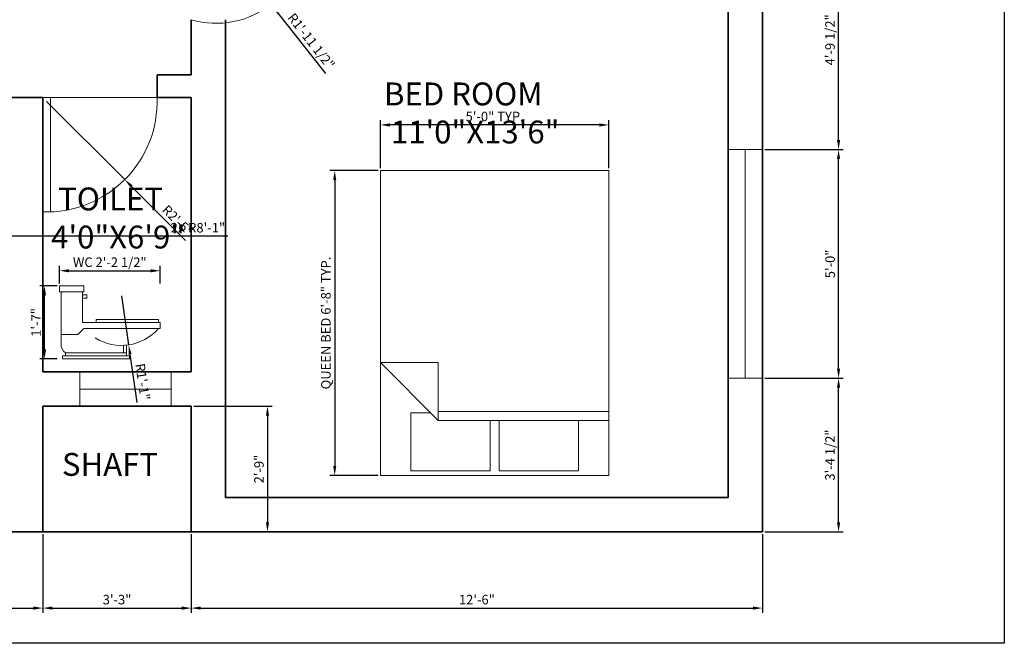
# Model space of a CAD drawing. Units: inches. Extents: x 5717 to 6221, y 11359 to 11763.
# Tile 3 of 4: x 5963 to 6221, y 11382 to 11546. Entities that reach past the tile are written whole.
import ezdxf

# ---------------------------------------------------------------- set-up
doc = ezdxf.new("R2010")
doc.units = ezdxf.units.IN
for name, color, linetype, lineweight, true_color in [('A-ANNO-DIMS', 254, 'Continuous', 13, 0xfeeab9), ('A-ANNO-TTLB', 51, 'Continuous', 25, 0xf8f6b0), ('A-AREA-IDEN', 11, 'Continuous', 20, 0xf27172), ('A-WALL', 244, 'Continuous', 35, 0x991b1e)]:
    doc.layers.add(name, color=color, linetype=linetype, lineweight=lineweight, true_color=true_color)
for name, color, linetype, lineweight in [('A-DOOR', 5, 'Continuous', 18), ('A-FLOR-FIXT', 1, 'Continuous', 18), ('A-FURN', 8, 'Continuous', 18), ('A-GLAZ', 4, 'Continuous', 18)]:
    doc.layers.add(name, color=color, linetype=linetype, lineweight=lineweight)
doc.styles.get("Standard").update_dxf_attribs({"font": 'arial.ttf'})
doc.dimstyles.new('ISO-25', dxfattribs={"dimtxt": 2.5, "dimasz": 2.5, "dimexe": 1.25, "dimexo": 0.625, "dimtad": 1, "dimlunit": 3, "dimtxsty": 'Standard', "dimcen": 2.5, "dimadec": 0, "dimazin": 0, "dimtfac": 1, "dimtmove": 0, "dimatfit": 3, "dimfxl": 1, "dimarcsym": 0})

# ---------------------------------------------------------------- blocks, each defined once
blk = doc.blocks.new('Toilet - side')
for p, q in [((0.5, 5), (0.5, 22)), ((7.5, 22), (7.5, 12)), ((7.5, 21), (9, 21)), ((9, 20), (7.5, 20)), ((9, 21), (9, 20)), ((32.5, 13), (12, 13)), ((12, 13), (12, 12)), ((32.5, 12), (32.5, 13)), ((8, 10), (6, 8)), ((7.5, 12), (33, 12)), ((33, 10), (8, 10)), ((33, 12), (33, 10)), ((6, 8), (0.5, 8)), ((21, 4.5), (21, 2)), ((22, 2), (22, 4.54)), ((22, 2), (2, 2)), ((2, 2), (2, 1)), ((22, 1), (22, 2))]:
    blk.add_line(p, q)
for points in [[(0, 22), (0, 24), (8, 24), (8, 22)], [(1, 0), (1, 1), (23, 1), (23, 0)]]:
    blk.add_lwpolyline(points, close=True)
for centre, radius, start, end in [((20.3, 20.7), 16.23, 238.1872, 318.7702), ((3.75, 4.75), 3.26, 175.6013, 237.5288)]:
    blk.add_arc(centre, radius, start, end)
blk = doc.blocks.new('Bed - Queen')
for p, q in [((0, -80.00003), (0, 0)), ((0, 0), (59.99999, 0)), ((59.99999, 0), (59.99999, -80.00003)), ((7.99999, -1.2), (28.79998, -1.2)), ((7.99999, -14.4), (7.99999, -1.2)), ((28.79998, -1.2), (28.79998, -14.4)), ((31.19999, -1.2), (51.99999, -1.2)), ((31.19999, -14.4), (31.19999, -1.2)), ((51.99999, -1.2), (51.99999, -16.4)), ((0, -14.4), (44.8, -14.4)), ((59.99999, -29.6), (44.8, -14.4)), ((44.8, -14.4), (44.8, -29.6)), ((44.8, -16.8), (0, -16.8)), ((51.99999, -16.4), (46.79936, -16.4)), ((44.8, -29.6), (59.99999, -29.6)), ((59.99999, -80.00003), (0, -80.00003))]:
    blk.add_line(p, q)
blk = doc.blocks.new('DOOR-LEAF-30IN')
for p, q in [((2, 30), (0, 30)), ((0, 30), (0, 0)), ((2, 0), (2, 30))]:
    blk.add_line(p, q)
blk = doc.blocks.new('WIN-24IN')
for p, q in [((0, 9), (0, 0)), ((24, 9), (0, 9)), ((24, 9), (24, 0)), ((24, 0), (24, 9)), ((0, 4.5), (24, 4.5)), ((0, 0), (24, 0))]:
    blk.add_line(p, q)
blk = doc.blocks.new('*D20')
at = {"layer": 'A-ANNO-DIMS', "color": 0, "lineweight": -2, "transparency": 16777216}
for p, q in [((6056.94, 11505.95), (6044.32, 11505.95)), ((6045.57, 11503.45), (6045.57, 11428.45)), ((6056.94, 11425.95), (6044.32, 11425.95))]:
    blk.add_line(p, q, dxfattribs=at)
at = {"layer": 'A-ANNO-DIMS', "color": 0, "transparency": 16777216}
for points in [[(6045.15, 11503.45), (6045.98, 11503.45), (6045.57, 11505.95)], [(6045.15, 11428.45), (6045.98, 11428.45), (6045.57, 11425.95)]]:
    blk.add_solid(points, dxfattribs=at)
at = {"layer": 'Defpoints', "color": 0, "transparency": 16777216}
for p in [(6057.57, 11505.95), (6045.57, 11425.95), (6057.57, 11425.95)]:
    blk.add_point(p, dxfattribs=at)
at = {"layer": 'A-ANNO-DIMS', "color": 0, "transparency": 16777216, "insert": (6043.57, 11465.95), "char_height": 2.5, "attachment_point": 5, "rotation": 90}
blk.add_mtext('QUEEN BED 6\'-8" TYP.', dxfattribs=at)
blk = doc.blocks.new('*D21')
at = {"layer": 'A-ANNO-DIMS', "color": 0, "lineweight": -2, "transparency": 16777216}
for p, q in [((6057.57, 11506.58), (6057.57, 11519.2)), ((6117.57, 11506.58), (6117.57, 11519.2)), ((6115.07, 11517.95), (6060.07, 11517.95))]:
    blk.add_line(p, q, dxfattribs=at)
at = {"layer": 'A-ANNO-DIMS', "color": 0, "transparency": 16777216}
for points in [[(6060.07, 11518.37), (6060.07, 11517.53), (6057.57, 11517.95)], [(6115.07, 11518.37), (6115.07, 11517.53), (6117.57, 11517.95)]]:
    blk.add_solid(points, dxfattribs=at)
at = {"layer": 'Defpoints', "color": 0, "transparency": 16777216}
for p in [(6057.57, 11517.95), (6057.57, 11505.95), (6117.57, 11505.95)]:
    blk.add_point(p, dxfattribs=at)
at = {"layer": 'A-ANNO-DIMS', "color": 0, "transparency": 16777216, "insert": (6087.57, 11519.85), "char_height": 2.5, "attachment_point": 5}
blk.add_mtext('5\'-0" TYP.', dxfattribs=at)
blk = doc.blocks.new('*D28')
at = {"layer": 'A-ANNO-DIMS', "color": 0, "lineweight": -2, "transparency": 16777216}
for p, q in [((5973.29, 11476.33), (5973.29, 11480.92)), ((5975.79, 11479.67), (5997.19, 11479.67)), ((5999.69, 11476.33), (5999.69, 11480.92))]:
    blk.add_line(p, q, dxfattribs=at)
at = {"layer": 'A-ANNO-DIMS', "color": 0, "transparency": 16777216}
for points in [[(5975.79, 11480.08), (5975.79, 11479.25), (5973.29, 11479.67)], [(5997.19, 11480.08), (5997.19, 11479.25), (5999.69, 11479.67)]]:
    blk.add_solid(points, dxfattribs=at)
at = {"layer": 'Defpoints', "color": 0, "transparency": 16777216}
for p in [(5999.69, 11479.67), (5973.29, 11475.71), (5999.69, 11475.71)]:
    blk.add_point(p, dxfattribs=at)
at = {"layer": 'A-ANNO-DIMS', "color": 0, "transparency": 16777216, "insert": (5986.49, 11481.58), "char_height": 2.5, "attachment_point": 5}
blk.add_mtext('WC 2\'-2 1/2"', dxfattribs=at)
blk = doc.blocks.new('*D29')
at = {"layer": 'A-ANNO-DIMS', "color": 0, "lineweight": -2, "transparency": 16777216}
for p, q in [((5972.67, 11475.71), (5968.08, 11475.71)), ((5969.33, 11459.01), (5969.33, 11473.21)), ((5972.67, 11456.51), (5968.08, 11456.51))]:
    blk.add_line(p, q, dxfattribs=at)
at = {"layer": 'A-ANNO-DIMS', "color": 0, "transparency": 16777216}
for points in [[(5968.92, 11473.21), (5969.75, 11473.21), (5969.33, 11475.71)], [(5968.92, 11459.01), (5969.75, 11459.01), (5969.33, 11456.51)]]:
    blk.add_solid(points, dxfattribs=at)
at = {"layer": 'Defpoints', "color": 0, "transparency": 16777216}
for p in [(5969.33, 11475.71), (5973.29, 11475.71), (5973.29, 11456.51)]:
    blk.add_point(p, dxfattribs=at)
at = {"layer": 'A-ANNO-DIMS', "color": 0, "transparency": 16777216, "insert": (5967.45, 11466.11), "char_height": 2.5, "attachment_point": 5, "rotation": 90}
blk.add_mtext('1\'-7"', dxfattribs=at)
blk = doc.blocks.new('*D38')
at = {"layer": 'A-ANNO-DIMS', "color": 0, "lineweight": -2, "transparency": 16777216}
for p, q in [((5797.9, 11410.48), (5797.9, 11389.86)), ((5968.9, 11410.48), (5968.9, 11389.86)), ((5800.4, 11391.11), (5966.4, 11391.11))]:
    blk.add_line(p, q, dxfattribs=at)
at = {"layer": 'A-ANNO-DIMS', "color": 0, "transparency": 16777216}
for points in [[(5800.4, 11391.53), (5800.4, 11390.69), (5797.9, 11391.11)], [(5966.4, 11391.53), (5966.4, 11390.69), (5968.9, 11391.11)]]:
    blk.add_solid(points, dxfattribs=at)
at = {"layer": 'Defpoints', "color": 0, "transparency": 16777216}
for p in [(5797.9, 11411.11), (5968.9, 11411.11), (5968.9, 11391.11)]:
    blk.add_point(p, dxfattribs=at)
at = {"layer": 'A-ANNO-DIMS', "color": 0, "transparency": 16777216, "insert": (5883.4, 11393.01), "char_height": 2.5, "attachment_point": 5}
blk.add_mtext('14\'-3"', dxfattribs=at)
blk = doc.blocks.new('*D39')
at = {"layer": 'A-ANNO-DIMS', "color": 0, "lineweight": -2, "transparency": 16777216}
for p, q in [((5968.9, 11410.48), (5968.9, 11389.86)), ((6007.9, 11410.48), (6007.9, 11389.86)), ((5971.4, 11391.11), (6005.4, 11391.11))]:
    blk.add_line(p, q, dxfattribs=at)
at = {"layer": 'A-ANNO-DIMS', "color": 0, "transparency": 16777216}
for points in [[(5971.4, 11391.53), (5971.4, 11390.69), (5968.9, 11391.11)], [(6005.4, 11391.53), (6005.4, 11390.69), (6007.9, 11391.11)]]:
    blk.add_solid(points, dxfattribs=at)
at = {"layer": 'Defpoints', "color": 0, "transparency": 16777216}
for p in [(5968.9, 11411.11), (6007.9, 11411.11), (6007.9, 11391.11)]:
    blk.add_point(p, dxfattribs=at)
at = {"layer": 'A-ANNO-DIMS', "color": 0, "transparency": 16777216, "insert": (5988.4, 11393.01), "char_height": 2.5, "attachment_point": 5}
blk.add_mtext('3\'-3"', dxfattribs=at)
blk = doc.blocks.new('*D40')
at = {"layer": 'A-ANNO-DIMS', "color": 0, "lineweight": -2, "transparency": 16777216}
for p, q in [((6007.9, 11410.48), (6007.9, 11389.86)), ((6157.9, 11410.48), (6157.9, 11389.86)), ((6010.4, 11391.11), (6155.4, 11391.11))]:
    blk.add_line(p, q, dxfattribs=at)
at = {"layer": 'A-ANNO-DIMS', "color": 0, "transparency": 16777216}
for points in [[(6010.4, 11391.53), (6010.4, 11390.69), (6007.9, 11391.11)], [(6155.4, 11391.53), (6155.4, 11390.69), (6157.9, 11391.11)]]:
    blk.add_solid(points, dxfattribs=at)
at = {"layer": 'Defpoints', "color": 0, "transparency": 16777216}
for p in [(6007.9, 11411.11), (6157.9, 11411.11), (6157.9, 11391.11)]:
    blk.add_point(p, dxfattribs=at)
at = {"layer": 'A-ANNO-DIMS', "color": 0, "transparency": 16777216, "insert": (6082.9, 11393.01), "char_height": 2.5, "attachment_point": 5}
blk.add_mtext('12\'-6"', dxfattribs=at)
blk = doc.blocks.new('*D41')
at = {"layer": 'A-ANNO-DIMS', "color": 0, "lineweight": -2, "transparency": 16777216}
for p, q in [((6158.53, 11451.47), (6179.15, 11451.47)), ((6177.9, 11413.61), (6177.9, 11448.97)), ((6158.53, 11411.11), (6179.15, 11411.11))]:
    blk.add_line(p, q, dxfattribs=at)
at = {"layer": 'A-ANNO-DIMS', "color": 0, "transparency": 16777216}
for points in [[(6177.49, 11448.97), (6178.32, 11448.97), (6177.9, 11451.47)], [(6177.49, 11413.61), (6178.32, 11413.61), (6177.9, 11411.11)]]:
    blk.add_solid(points, dxfattribs=at)
at = {"layer": 'Defpoints', "color": 0, "transparency": 16777216}
for p in [(6157.9, 11451.47), (6177.9, 11451.47), (6157.9, 11411.11)]:
    blk.add_point(p, dxfattribs=at)
at = {"layer": 'A-ANNO-DIMS', "color": 0, "transparency": 16777216, "insert": (6175.98, 11431.29), "char_height": 2.5, "attachment_point": 5, "rotation": 90}
blk.add_mtext('3\'-4 1/2"', dxfattribs=at)
blk = doc.blocks.new('*D42')
at = {"layer": 'A-ANNO-DIMS', "color": 0, "lineweight": -2, "transparency": 16777216}
for p, q in [((6158.53, 11511.47), (6179.15, 11511.47)), ((6177.9, 11453.97), (6177.9, 11508.97)), ((6158.53, 11451.47), (6179.15, 11451.47))]:
    blk.add_line(p, q, dxfattribs=at)
at = {"layer": 'A-ANNO-DIMS', "color": 0, "transparency": 16777216}
for points in [[(6177.49, 11508.97), (6178.32, 11508.97), (6177.9, 11511.47)], [(6177.49, 11453.97), (6178.32, 11453.97), (6177.9, 11451.47)]]:
    blk.add_solid(points, dxfattribs=at)
at = {"layer": 'Defpoints', "color": 0, "transparency": 16777216}
for p in [(6157.9, 11511.47), (6177.9, 11511.47), (6157.9, 11451.47)]:
    blk.add_point(p, dxfattribs=at)
at = {"layer": 'A-ANNO-DIMS', "color": 0, "transparency": 16777216, "insert": (6176, 11481.47), "char_height": 2.5, "attachment_point": 5, "rotation": 90}
blk.add_mtext('5\'-0"', dxfattribs=at)
blk = doc.blocks.new('*D43')
at = {"layer": 'A-ANNO-DIMS', "color": 0, "lineweight": -2, "transparency": 16777216}
for p, q in [((6158.53, 11569.11), (6179.15, 11569.11)), ((6177.9, 11513.97), (6177.9, 11566.61)), ((6158.53, 11511.47), (6179.15, 11511.47))]:
    blk.add_line(p, q, dxfattribs=at)
at = {"layer": 'A-ANNO-DIMS', "color": 0, "transparency": 16777216}
for points in [[(6177.49, 11566.61), (6178.32, 11566.61), (6177.9, 11569.11)], [(6177.49, 11513.97), (6178.32, 11513.97), (6177.9, 11511.47)]]:
    blk.add_solid(points, dxfattribs=at)
at = {"layer": 'Defpoints', "color": 0, "transparency": 16777216}
for p in [(6157.9, 11569.11), (6177.9, 11569.11), (6157.9, 11511.47)]:
    blk.add_point(p, dxfattribs=at)
at = {"layer": 'A-ANNO-DIMS', "color": 0, "transparency": 16777216, "insert": (6175.98, 11540.29), "char_height": 2.5, "attachment_point": 5, "rotation": 90}
blk.add_mtext('4\'-9 1/2"', dxfattribs=at)
blk = doc.blocks.new('*D57')
at = {"layer": 'A-ANNO-DIMS', "color": 0, "lineweight": -2, "transparency": 16777216}
for p, q in [((6008.53, 11444.11), (6029.15, 11444.11)), ((6027.9, 11441.61), (6027.9, 11413.61)), ((6008.53, 11411.11), (6029.15, 11411.11))]:
    blk.add_line(p, q, dxfattribs=at)
at = {"layer": 'A-ANNO-DIMS', "color": 0, "transparency": 16777216}
for points in [[(6027.49, 11441.61), (6028.32, 11441.61), (6027.9, 11444.11)], [(6027.49, 11413.61), (6028.32, 11413.61), (6027.9, 11411.11)]]:
    blk.add_solid(points, dxfattribs=at)
at = {"layer": 'Defpoints', "color": 0, "transparency": 16777216}
for p in [(6007.9, 11444.11), (6007.9, 11411.11), (6027.9, 11411.11)]:
    blk.add_point(p, dxfattribs=at)
at = {"layer": 'A-ANNO-DIMS', "color": 0, "transparency": 16777216, "insert": (6026, 11427.61), "char_height": 2.5, "attachment_point": 5, "rotation": 90}
blk.add_mtext('2\'-9"', dxfattribs=at)
blk = doc.blocks.new('*D64')
at = {"layer": 'A-ANNO-DIMS', "color": 0, "lineweight": -2, "transparency": 16777216}
for p, q in [((5969.9, 11524.11), (5990.42, 11503.59)), ((6006.37, 11487.64), (5992.19, 11501.82))]:
    blk.add_line(p, q, dxfattribs=at)
at = {"layer": 'A-ANNO-DIMS', "color": 0, "transparency": 16777216}
blk.add_solid([(5992.48, 11502.12), (5991.89, 11501.53), (5990.42, 11503.59)], dxfattribs=at)
at = {"layer": 'Defpoints', "color": 0, "transparency": 16777216}
for p in [(5969.9, 11524.11), (5990.42, 11503.59)]:
    blk.add_point(p, dxfattribs=at)
at = {"layer": 'A-ANNO-DIMS', "color": 0, "transparency": 16777216, "insert": (6004.08, 11492.62), "char_height": 2.5, "attachment_point": 5, "rotation": 315.0011}
blk.add_mtext('R2\'-5"', dxfattribs=at)
blk = doc.blocks.new('*D66')
at = {"layer": 'A-ANNO-DIMS', "color": 0, "lineweight": -2, "transparency": 16777216}
for p, q in [((6014.46, 11568.11), (6028.94, 11549.64)), ((6043.2, 11531.46), (6030.48, 11547.68))]:
    blk.add_line(p, q, dxfattribs=at)
at = {"layer": 'A-ANNO-DIMS', "color": 0, "transparency": 16777216}
blk.add_solid([(6030.81, 11547.93), (6030.16, 11547.42), (6028.94, 11549.64)], dxfattribs=at)
at = {"layer": 'Defpoints', "color": 0, "transparency": 16777216}
for p in [(6014.46, 11568.11), (6028.94, 11549.64)]:
    blk.add_point(p, dxfattribs=at)
at = {"layer": 'A-ANNO-DIMS', "color": 0, "transparency": 16777216, "insert": (6039.14, 11539.75), "char_height": 2.5, "attachment_point": 5, "rotation": 308.1145}
blk.add_mtext('R1\'-11 1/2"', dxfattribs=at)
blk = doc.blocks.new('*D67')
at = {"layer": 'A-ANNO-DIMS', "color": 0, "lineweight": -2, "transparency": 16777216}
for p, q in [((5854.49, 11488.73), (5951.44, 11488.73)), ((6017.47, 11488.73), (5953.94, 11488.73))]:
    blk.add_line(p, q, dxfattribs=at)
at = {"layer": 'A-ANNO-DIMS', "color": 0, "transparency": 16777216}
blk.add_solid([(5953.94, 11489.15), (5953.94, 11488.32), (5951.44, 11488.73)], dxfattribs=at)
at = {"layer": 'Defpoints', "color": 0, "transparency": 16777216}
for p in [(5854.49, 11488.73), (5951.44, 11488.73)]:
    blk.add_point(p, dxfattribs=at)
at = {"layer": 'A-ANNO-DIMS', "color": 0, "transparency": 16777216, "insert": (6009.62, 11490.64), "char_height": 2.5, "attachment_point": 5, "rotation": 360}
blk.add_mtext('2X R8\'-1"', dxfattribs=at)
blk = doc.blocks.new('*D69')
at = {"layer": 'A-ANNO-DIMS', "color": 0, "lineweight": -2, "transparency": 16777216}
for p, q in [((5989.53, 11473.06), (5991.44, 11460.22)), ((5993.7, 11445.1), (5991.81, 11457.75))]:
    blk.add_line(p, q, dxfattribs=at)
at = {"layer": 'A-ANNO-DIMS', "color": 0, "transparency": 16777216}
blk.add_solid([(5992.22, 11457.81), (5991.4, 11457.69), (5991.44, 11460.22)], dxfattribs=at)
at = {"layer": 'Defpoints', "color": 0, "transparency": 16777216}
for p in [(5989.53, 11473.06), (5991.44, 11460.22)]:
    blk.add_point(p, dxfattribs=at)
at = {"layer": 'A-ANNO-DIMS', "color": 0, "transparency": 16777216, "insert": (5994.8, 11450.47), "char_height": 2.5, "attachment_point": 5, "rotation": 278.4771}
blk.add_mtext('R1\'-1"', dxfattribs=at)

msp = doc.modelspace()

# ---------------------------------------------------------------- linework, layer by layer
at = {"layer": 'A-ANNO-TTLB'}
msp.add_lwpolyline([(5717.423, 11763.126), (6221.432, 11763.126), (6221.432, 11381.867), (5717.423, 11381.867)], close=True, dxfattribs=at)
at = {"layer": 'A-DOOR'}
for p, q in [((5968.902, 11525.109), (5998.902, 11525.109)), ((5998.902, 11525.109), (5968.902, 11525.109))]:
    msp.add_line(p, q, dxfattribs=at)
for centre, radius, start, end in [((6014.455, 11568.109), 23.469, 253.78655, 2.44213), ((5969.902, 11524.109), 29.017, 268.02507, 1.97493)]:
    msp.add_arc(centre, radius, start, end, dxfattribs=at)
at = {"layer": 'A-GLAZ'}
for p, q in [((6148.902, 11451.47), (6148.902, 11511.47)), ((6157.902, 11511.47), (6148.902, 11511.47)), ((6153.402, 11451.47), (6153.402, 11511.47)), ((6157.902, 11451.47), (6157.902, 11511.47)), ((6148.902, 11451.47), (6157.902, 11451.47))]:
    msp.add_line(p, q, dxfattribs=at)
at = {"layer": 'A-WALL'}
for p, q in [((6157.902, 11411.109), (6157.902, 11711.109)), ((6148.902, 11420.109), (6148.902, 11569.109)), ((6007.902, 11531.109), (6007.902, 11545.574)), ((6016.902, 11420.109), (6016.902, 11545.574)), ((5998.902, 11531.109), (6007.902, 11531.109)), ((5998.902, 11525.109), (5998.902, 11531.109)), ((5959.902, 11525.109), (5968.902, 11525.109)), ((5968.902, 11453.109), (5968.902, 11525.109)), ((5998.902, 11525.109), (6007.902, 11525.109)), ((6007.902, 11453.109), (6007.902, 11525.109)), ((5968.902, 11453.109), (6007.902, 11453.109)), ((5968.902, 11411.109), (5968.902, 11444.109)), ((5968.902, 11444.109), (6007.902, 11444.109)), ((6007.902, 11411.109), (6007.902, 11444.109)), ((6016.902, 11420.109), (6148.902, 11420.109)), ((5797.902, 11411.109), (6157.902, 11411.109))]:
    msp.add_line(p, q, dxfattribs=at)

# ---------------------------------------------------------------- block references
at = {"layer": 'A-DOOR', "rotation": 180}
msp.add_blockref('DOOR-LEAF-30IN', (5970.902, 11525.109), dxfattribs=at)
at = {"layer": 'A-FLOR-FIXT', "xscale": 0.8, "yscale": 0.8, "zscale": 0.8}
msp.add_blockref('Toilet - side', (5973.293, 11456.506), dxfattribs=at)
at = {"layer": 'A-FURN', "rotation": 180}
msp.add_blockref('Bed - Queen', (6117.568, 11425.95), dxfattribs=at)
at = {"layer": 'A-GLAZ'}
msp.add_blockref('WIN-24IN', (5978.601, 11444.109), dxfattribs=at)

# ---------------------------------------------------------------- texts
at = {"layer": 'A-AREA-IDEN', "char_height": 6, "attachment_point": 1}
for s, insert in [('     BED ROOM\\P      11\'0"X13\'6"', (6049.33, 11529.088)), (' TOILET\\P4\'0"X6\'9"', (5971.091, 11501.517)), ('  SHAFT', (5970.26, 11431.829))]:
    msp.add_mtext_dynamic_manual_height_columns(s, width=116.60264, gutter_width=12.5, heights=[0], dxfattribs=dict(at, insert=insert))

# ---------------------------------------------------------------- dimensions: what is measured, and where the dimension line sits
at = {"layer": 'A-ANNO-DIMS'}
for center, mpoint, picture, middle in [((6014.455, 11568.109), (6028.941, 11549.644), '*D66', (6037.632, 11538.566)), ((5969.902, 11524.109), (5990.421, 11503.591), '*D64', (6002.732, 11491.28))]:
    dim = msp.add_radius_dim(center=center, mpoint=mpoint, dimstyle='ISO-25', override={"dimdec": 1, "dimlfac": 1, "dimrnd": 0, "dimzin": 1, "dimdsep": 46, "dimlunit": 4, "dimfrac": 2}, dxfattribs=at)
    dim.commit()
    dim.dimension.update_dxf_attribs({"geometry": picture, "text_midpoint": middle, "dimtype": 164})
for base, p1, p2, angle, picture, middle in [((6177.902, 11569.109), (6157.902, 11511.47), (6157.902, 11569.109), 90, '*D43', (6175.985, 11540.29)), ((6177.902, 11511.47), (6157.902, 11451.47), (6157.902, 11511.47), 90, '*D42', (6176.001, 11481.47)), ((5969.333, 11475.706), (5973.293, 11456.506), (5973.293, 11475.706), 90, '*D29', (5967.453, 11466.106)), ((6177.902, 11451.47), (6157.902, 11411.109), (6157.902, 11451.47), 90, '*D41', (6175.984, 11431.29)), ((6027.902, 11411.109), (6007.902, 11444.109), (6007.902, 11411.109), 270, '*D57', (6026.001, 11427.609))]:
    dim = msp.add_linear_dim(base=base, p1=p1, p2=p2, angle=angle, dimstyle='ISO-25', override={"dimdec": 1, "dimlfac": 1, "dimrnd": 0, "dimzin": 1, "dimdsep": 46, "dimlunit": 4, "dimfrac": 2}, dxfattribs=at)
    dim.commit()
    dim.dimension.update_dxf_attribs({"geometry": picture, "text_midpoint": middle})
for base, p1, p2, angle, text, picture, middle in [((6057.568, 11517.95), (6117.568, 11505.95), (6057.568, 11505.95), 180, '<> TYP.', '*D21', (6087.568, 11519.852)), ((6045.568, 11425.95), (6057.568, 11505.95), (6057.568, 11425.95), 270, 'QUEEN BED <> TYP.', '*D20', (6043.573, 11465.95))]:
    dim = msp.add_linear_dim(base=base, p1=p1, p2=p2, angle=angle, text=text, dimstyle='ISO-25', override={"dimdec": 1, "dimlfac": 1, "dimrnd": 0, "dimzin": 1, "dimdsep": 46, "dimlunit": 4, "dimfrac": 2}, dxfattribs=at)
    dim.commit()
    dim.dimension.update_dxf_attribs({"geometry": picture, "text_midpoint": middle})
dim = msp.add_radius_dim(center=(5854.485, 11488.735), mpoint=(5951.443, 11488.735), text='2X <>', dimstyle='ISO-25', override={"dimdec": 1, "dimlfac": 1, "dimrnd": 0, "dimzin": 1, "dimdsep": 46, "dimlunit": 4, "dimfrac": 2}, dxfattribs=at)
dim.commit()
dim.dimension.update_dxf_attribs({"geometry": '*D67', "text_midpoint": (6009.617, 11488.735), "dimtype": 164})
dim = msp.add_linear_dim(base=(5999.693, 11479.666), p1=(5973.293, 11475.706), p2=(5999.693, 11475.706), text='WC <>', dimstyle='ISO-25', override={"dimdec": 1, "dimlfac": 1, "dimrnd": 0, "dimzin": 1, "dimdsep": 46, "dimlunit": 4, "dimfrac": 2}, dxfattribs=at)
dim.commit()
dim.dimension.update_dxf_attribs({"geometry": '*D28', "text_midpoint": (5986.493, 11481.583)})
dim = msp.add_radius_dim(center=(5989.529, 11473.062), mpoint=(5991.443, 11460.221), dimstyle='ISO-25', override={"dimdec": 1, "dimlfac": 1, "dimrnd": 0, "dimzin": 1, "dimdsep": 46, "dimlunit": 4, "dimfrac": 2}, dxfattribs=at)
dim.commit()
dim.dimension.update_dxf_attribs({"geometry": '*D69', "text_midpoint": (5994.798, 11450.465)})
for base, p1, p2, picture, middle in [((5968.902, 11391.109), (5797.902, 11411.109), (5968.902, 11411.109), '*D38', (5883.402, 11393.011)), ((6007.902, 11391.109), (5968.902, 11411.109), (6007.902, 11411.109), '*D39', (5988.402, 11393.011)), ((6157.902, 11391.109), (6007.902, 11411.109), (6157.902, 11411.109), '*D40', (6082.902, 11393.01))]:
    dim = msp.add_linear_dim(base=base, p1=p1, p2=p2, dimstyle='ISO-25', override={"dimdec": 1, "dimlfac": 1, "dimrnd": 0, "dimzin": 1, "dimdsep": 46, "dimlunit": 4, "dimfrac": 2}, dxfattribs=at)
    dim.commit()
    dim.dimension.update_dxf_attribs({"geometry": picture, "text_midpoint": middle})

doc.saveas('drawing.dxf')
